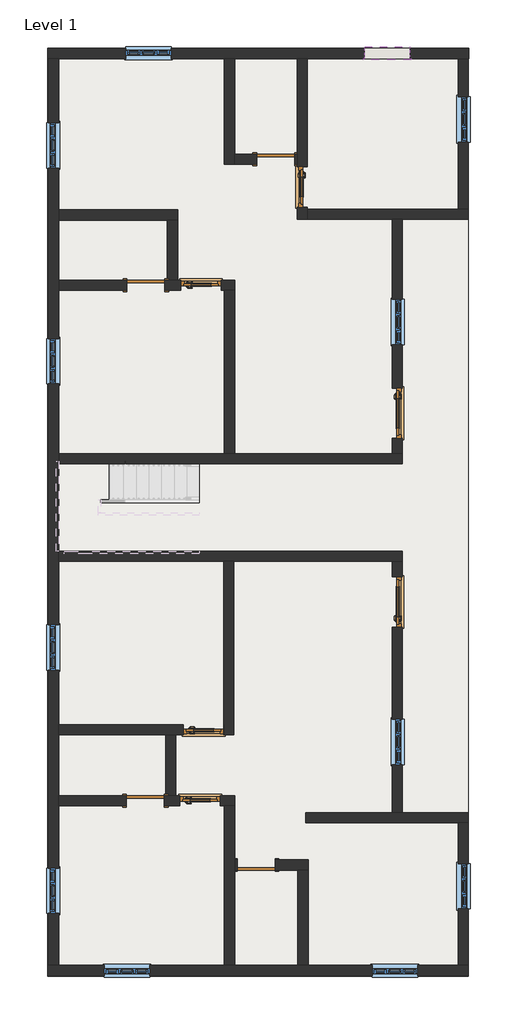
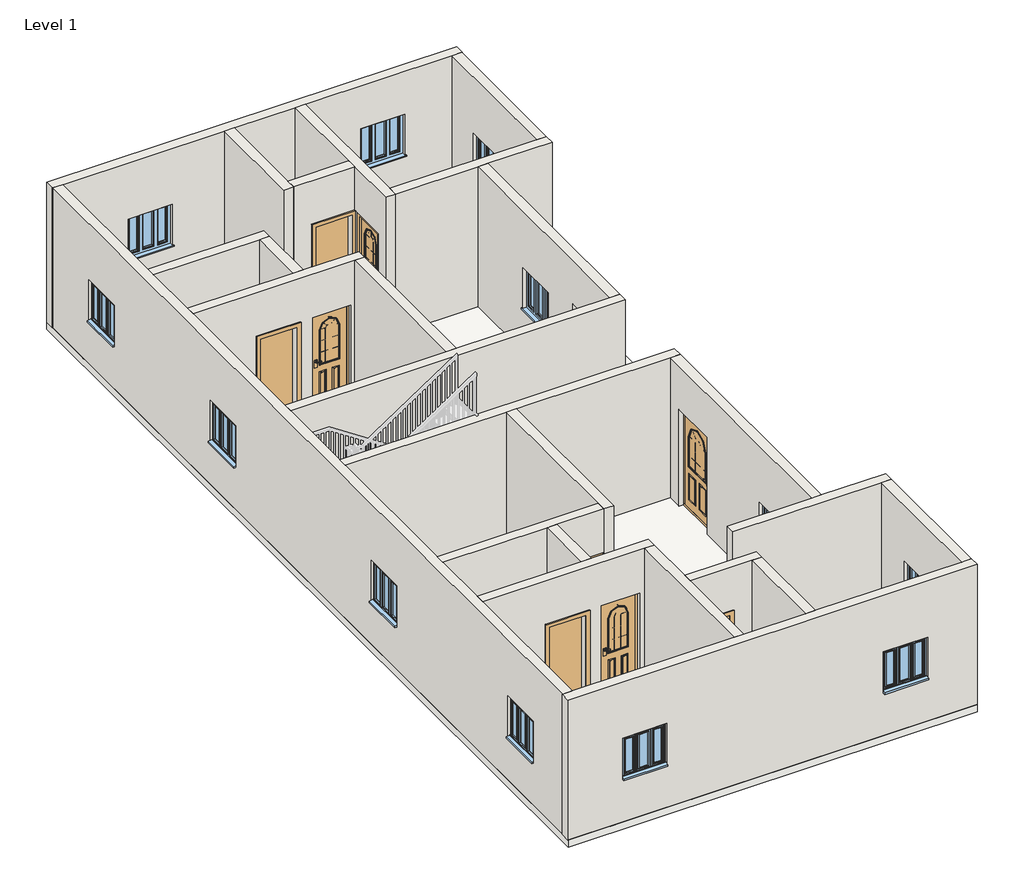
# One storey, part 1 of 2: 25 walls, 12 windows, 10 doors, 1 slab.
"""IFC4 building model written with IfcOpenShell, lengths in millimetres."""

from ifc_helpers import new_model, si_unit, frame, origin, origin_with_axes, place, context, project, spatial, polyline, outline, extrude, faceted_brep, transform, mapped, element, save
from components import doors_extsgl_w_glazing_bars_arched_1010x2110mm_bccdb1b2, doors_extsgl_w_glazing_bars_arched_1010x2110mm_5c897e1f, doors_extsgl_w_glazing_bars_arched_810x2110mm_57ea6d9e, doors_extsgl_w_glazing_bars_arched_810x2110mm_84a0a083, door_fadea3f2, windows_tpl_w_glazing_bars_910x910mm_9d987a72

model = new_model("IFC4")

# Units and contexts
model_context = context("Model", 3, world=origin())
ifc_project = project(units=[si_unit("LENGTHUNIT", "METRE", prefix="MILLI")], contexts=[model_context])

# Site, building, storey
site = spatial("IfcSite", under=ifc_project)
building = spatial("IfcBuilding", under=site)
storey = spatial("IfcBuildingStorey", under=building, Name="Level 1", Elevation=0.0)

# Doors
placement = place(None, origin())
doors_extsgl_w_glazing_bars_arched_1010x2110mm_shape = doors_extsgl_w_glazing_bars_arched_1010x2110mm_bccdb1b2(model_context)
element("IfcDoor", 1, ObjectType="Doors_ExtSgl_w-Glazing_Bars_Arched : 1010x2110mm", at=placement, inside=storey, context=model_context, shape_type="MappedRepresentation", body=[
    mapped(doors_extsgl_w_glazing_bars_arched_1010x2110mm_shape, transform((1850.5605895, 2208.5797121, 0.0), x_axis=(0.0, -1.0, 0.0), y_axis=(1.0, 0.0, 0.0), z_axis=(0.0, 0.0, 1.0))),
])
doors_extsgl_w_glazing_bars_arched_1010x2110mm_2_shape = doors_extsgl_w_glazing_bars_arched_1010x2110mm_5c897e1f(model_context)
element("IfcDoor", 2, ObjectType="Doors_ExtSgl_w-Glazing_Bars_Arched : 1010x2110mm", at=placement, inside=storey, context=model_context, shape_type="MappedRepresentation", body=[
    mapped(doors_extsgl_w_glazing_bars_arched_1010x2110mm_2_shape, transform((1850.5605895, -1576.0202879, 0.0), x_axis=(0.0, 1.0, 0.0), y_axis=(-1.0, 0.0, 0.0), z_axis=(0.0, 0.0, 1.0))),
])
doors_extsgl_w_glazing_bars_arched_810x2110mm_shape = doors_extsgl_w_glazing_bars_arched_810x2110mm_57ea6d9e(model_context)
element("IfcDoor", 3, ObjectType="Doors_ExtSgl_w-Glazing_Bars_Arched : 810x2110mm", at=placement, inside=storey, context=model_context, shape_type="MappedRepresentation", body=[
    mapped(doors_extsgl_w_glazing_bars_arched_810x2110mm_shape, transform((-2086.4394105, 4773.9797121, 0.0), x_axis=(1.0, 0.0, 0.0), y_axis=(0.0, 1.0, 0.0), z_axis=(0.0, 0.0, 1.0))),
])
element("IfcDoor", 4, ObjectType="Doors_ExtSgl_w-Glazing_Bars_Arched : 810x2110mm", at=placement, inside=storey, context=model_context, shape_type="MappedRepresentation", body=[
    mapped(doors_extsgl_w_glazing_bars_arched_810x2110mm_shape, transform((-2105.4894105, -5563.8202879, 0.0), x_axis=(1.0, 0.0, 0.0), y_axis=(0.0, 1.0, 0.0), z_axis=(0.0, 0.0, 1.0))),
])
doors_extsgl_w_glazing_bars_arched_810x2110mm_2_shape = doors_extsgl_w_glazing_bars_arched_810x2110mm_84a0a083(model_context)
element("IfcDoor", 5, ObjectType="Doors_ExtSgl_w-Glazing_Bars_Arched : 810x2110mm", at=placement, inside=storey, context=model_context, shape_type="MappedRepresentation", body=[
    mapped(doors_extsgl_w_glazing_bars_arched_810x2110mm_2_shape, transform((-2035.6394105, -4141.4202879, 0.0), x_axis=(1.0, 0.0, 0.0), y_axis=(0.0, 1.0, 0.0), z_axis=(0.0, 0.0, 1.0))),
])
element("IfcDoor", 6, ObjectType="Doors_ExtSgl_w-Glazing_Bars_Arched : 810x2110mm", at=placement, inside=storey, context=model_context, shape_type="MappedRepresentation", body=[
    mapped(doors_extsgl_w_glazing_bars_arched_810x2110mm_2_shape, transform((-54.4394105, 6748.5640518, 0.0), x_axis=(0.0, -1.0, 0.0), y_axis=(1.0, 0.0, 0.0), z_axis=(0.0, 0.0, 1.0))),
])
door_shape = door_fadea3f2(model_context)
element("IfcDoor", 7, ObjectType="Single-Flush : 30\" x 80\"", at=placement, inside=storey, context=model_context, shape_type="MappedRepresentation", body=[
    mapped(door_shape, transform((-3204.0394105, -5563.8202879, 0.0), x_axis=(1.0, 0.0, 0.0), y_axis=(0.0, 1.0, 0.0), z_axis=(0.0, 0.0, 1.0))),
])
element("IfcDoor", 8, ObjectType="Single-Flush : 30\" x 80\"", at=placement, inside=storey, context=model_context, shape_type="MappedRepresentation", body=[
    mapped(door_shape, transform((-981.5394105, -6850.9128362, 0.0), x_axis=(-1.0, 0.0, 0.0), y_axis=(0.0, -1.0, 0.0), z_axis=(0.0, 0.0, 1.0))),
])
element("IfcDoor", 9, ObjectType="Single-Flush : 30\" x 80\"", at=placement, inside=storey, context=model_context, shape_type="MappedRepresentation", body=[
    mapped(door_shape, transform((-3191.3394105, 4773.9797121, 0.0), x_axis=(1.0, 0.0, 0.0), y_axis=(0.0, 1.0, 0.0), z_axis=(0.0, 0.0, 1.0))),
])
element("IfcDoor", 10, ObjectType="Single-Flush : 30\" x 80\"", at=placement, inside=storey, context=model_context, shape_type="MappedRepresentation", body=[
    mapped(door_shape, transform((-587.8394105, 7301.2797121, 0.0), x_axis=(1.0, 0.0, 0.0), y_axis=(0.0, 1.0, 0.0), z_axis=(0.0, 0.0, 1.0))),
])

# Slab
element("IfcSlab", 11, ObjectType="Generic - 12\"", at=placement, inside=storey, context=model_context, shape_type="SweptSolid", body=[
    extrude(outline(polyline([(3272.9605895, 9523.7797121), (3272.9605895, -9081.7202879), (-5159.8394105, -9081.7202879), (-5159.8394105, 9523.7797121), (3272.9605895, 9523.7797121)])), frame((0.0, 0.0, -152.4), z_axis=(0.0, 0.0, 1.0), x_axis=(1.0, 0.0, 0.0)), (0.0, 0.0, 1.0), 152.4),
])

# Walls
element("IfcWall", 12, ObjectType="Generic - 4.5\" p", at=placement, inside=storey, context=model_context, shape_type="Brep", body=[
    faceted_brep([(-2810.3394105, 4672.3797121, 2032.0), (-2810.3394105, 4672.3797121, 0.0), (-2491.4394105, 4672.3797121, 0.0), (-2491.4394105, 4672.3797121, 2110.0), (-1681.4394105, 4672.3797121, 2110.0), (-1681.4394105, 4672.3797121, 0.0), (-1616.5394105, 4672.3797121, 0.0), (-1413.3394105, 4672.3797121, 0.0), (-1413.3394105, 4672.3797121, 3048.0), (-1616.5394105, 4672.3797121, 3048.0), (-4943.9394105, 4672.3797121, 3048.0), (-4943.9394105, 4672.3797121, 0.0), (-3572.3394105, 4672.3797121, 0.0), (-3572.3394105, 4672.3797121, 2032.0), (-2491.4394105, 4875.5797121, 0.0), (-2556.3394105, 4875.5797121, 0.0), (-2759.5394105, 4875.5797121, 0.0), (-2810.3394105, 4875.5797121, 0.0), (-2810.3394105, 4875.5797121, 2032.0), (-3572.3394105, 4875.5797121, 2032.0), (-3572.3394105, 4875.5797121, 0.0), (-4943.9394105, 4875.5797121, 0.0), (-4943.9394105, 4875.5797121, 3048.0), (-2759.5394105, 4875.5797121, 3048.0), (-2556.3394105, 4875.5797121, 3048.0), (-1413.3394105, 4875.5797121, 3048.0), (-1413.3394105, 4875.5797121, 0.0), (-1681.4394105, 4875.5797121, 0.0), (-1681.4394105, 4875.5797121, 2110.0), (-2491.4394105, 4875.5797121, 2110.0)], [[[0, 1, 2, 3, 4, 5, 6, 7, 8, 9, 10, 11, 12, 13]], [[14, 15, 16, 17, 18, 19, 20, 21, 22, 23, 24, 25, 26, 27, 28, 29]], [[7, 6, 5, 27, 26]], [[12, 11, 21, 20]], [[2, 1, 17, 16, 15, 14]], [[10, 9, 8, 25, 24, 23, 22]], [[11, 10, 22, 21]], [[8, 7, 26, 25]], [[14, 29, 3, 2]], [[28, 27, 5, 4]], [[29, 28, 4, 3]], [[18, 17, 1, 0]], [[19, 18, 0, 13]], [[20, 19, 13, 12]]]),
])
element("IfcWall", 13, ObjectType="Generic - 4.5\" p", at=placement, inside=storey, context=model_context, shape_type="SweptSolid", body=[
    extrude(outline(polyline([(-1616.5394105, 1395.7797121), (-1616.5394105, 4672.3797121), (-1413.3394105, 4672.3797121), (-1413.3394105, 1395.7797121), (-1616.5394105, 1395.7797121)])), origin_with_axes(), (0.0, 0.0, 1.0), 3048.0),
])
element("IfcWall", 14, ObjectType="Generic - 4.5\" p", at=placement, inside=storey, context=model_context, shape_type="Brep", body=[
    faceted_brep([(-4943.9394105, 6082.1542467, 0.0), (-2759.5394105, 6082.1542467, 0.0), (-2556.3394105, 6082.1542467, 0.0), (-2556.3394105, 6082.1542467, 3048.0), (-2759.5394105, 6082.1542467, 3048.0), (-4943.9394105, 6082.1542467, 3048.0), (-4943.9394105, 6285.3542467, 0.0), (-4943.9394105, 6285.3542467, 3048.0), (-2556.3394105, 6285.3542467, 3048.0), (-2556.3394105, 6285.3542467, 0.0)], [[[0, 1, 2, 3, 4, 5]], [[6, 7, 8, 9]], [[2, 1, 0, 6, 9]], [[5, 4, 3, 8, 7]], [[0, 5, 7, 6]], [[3, 2, 9, 8]]]),
])
element("IfcWall", 15, ObjectType="Generic - 4.5\" p", at=placement, inside=storey, context=model_context, shape_type="SweptSolid", body=[
    extrude(outline(polyline([(-2759.5394105, 4875.5797121), (-2759.5394105, 6082.1542467), (-2556.3394105, 6082.1542467), (-2556.3394105, 4875.5797121), (-2759.5394105, 4875.5797121)])), origin_with_axes(), (0.0, 0.0, 1.0), 3048.0),
])
element("IfcWall", 16, ObjectType="Generic - 4.5\" p", at=placement, inside=storey, context=model_context, shape_type="Brep", body=[
    faceted_brep([(-1616.5394105, 9320.5797121, 0.0), (-1616.5394105, 7199.6797121, 0.0), (-1616.5394105, 7199.6797121, 3048.0), (-1616.5394105, 9320.5797121, 3048.0), (-1413.3394105, 9320.5797121, 0.0), (-1413.3394105, 9320.5797121, 3048.0), (-1413.3394105, 7402.8797121, 3048.0), (-1413.3394105, 7199.6797121, 3048.0), (-1413.3394105, 7199.6797121, 0.0), (-1413.3394105, 7402.8797121, 0.0)], [[[0, 1, 2, 3]], [[4, 5, 6, 7, 8, 9]], [[1, 0, 4, 9, 8]], [[3, 2, 7, 6, 5]], [[0, 3, 5, 4]], [[2, 1, 8, 7]]]),
])
element("IfcWall", 17, ObjectType="Generic - 4.5\" p", at=placement, inside=storey, context=model_context, shape_type="SweptSolid", body=[
    extrude(outline(polyline([(2032.0, -206.8394105), (0.0, -206.8394105), (0.0, -156.0394105), (3048.0, -156.0394105), (3048.0, -1413.3394105), (0.0, -1413.3394105), (0.0, -968.8394105), (2032.0, -968.8394105), (2032.0, -206.8394105)])), frame((0.0, 7199.6797121, 0.0), z_axis=(0.0, 1.0, 0.0), x_axis=(0.0, 0.0, 1.0)), (0.0, 0.0, 1.0), 203.2),
])
element("IfcWall", 18, ObjectType="Generic - 4.5\" p", at=placement, inside=storey, context=model_context, shape_type="Brep", body=[
    faceted_brep([(-156.0394105, 6343.5640518, 2110.0), (-156.0394105, 6343.5640518, 0.0), (-156.0394105, 6094.2483916, 0.0), (-156.0394105, 6094.2483916, 3048.0), (-156.0394105, 7199.6797121, 3048.0), (-156.0394105, 7402.8797121, 3048.0), (-156.0394105, 9320.5797121, 3048.0), (-156.0394105, 9320.5797121, 0.0), (-156.0394105, 7402.8797121, 0.0), (-156.0394105, 7199.6797121, 0.0), (-156.0394105, 7153.5640518, 0.0), (-156.0394105, 7153.5640518, 2110.0), (47.1605895, 6094.2483916, 0.0), (47.1605895, 6297.4483916, 0.0), (47.1605895, 6343.5640518, 0.0), (47.1605895, 6343.5640518, 2110.0), (47.1605895, 7153.5640518, 2110.0), (47.1605895, 7153.5640518, 0.0), (47.1605895, 9320.5797121, 0.0), (47.1605895, 9320.5797121, 3048.0), (47.1605895, 6297.4483916, 3048.0), (47.1605895, 6094.2483916, 3048.0)], [[[0, 1, 2, 3, 4, 5, 6, 7, 8, 9, 10, 11]], [[12, 13, 14, 15, 16, 17, 18, 19, 20, 21]], [[2, 1, 14, 13, 12]], [[10, 9, 8, 7, 18, 17]], [[6, 5, 4, 3, 21, 20, 19]], [[7, 6, 19, 18]], [[3, 2, 12, 21]], [[17, 16, 11, 10]], [[15, 14, 1, 0]], [[16, 15, 0, 11]]]),
])
element("IfcWall", 19, ObjectType="Generic - 4.5\" p", at=placement, inside=storey, context=model_context, shape_type="Brep", body=[
    faceted_brep([(47.1605895, 6094.2483916, 0.0), (1748.9605895, 6094.2483916, 0.0), (1952.1605895, 6094.2483916, 0.0), (3272.9605895, 6094.2483916, 0.0), (3272.9605895, 6094.2483916, 3048.0), (1952.1605895, 6094.2483916, 3048.0), (1748.9605895, 6094.2483916, 3048.0), (47.1605895, 6094.2483916, 3048.0), (47.1605895, 6297.4483916, 0.0), (47.1605895, 6297.4483916, 3048.0), (3069.7605895, 6297.4483916, 3048.0), (3272.9605895, 6297.4483916, 3048.0), (3272.9605895, 6297.4483916, 0.0), (3069.7605895, 6297.4483916, 0.0)], [[[0, 1, 2, 3, 4, 5, 6, 7]], [[8, 9, 10, 11, 12, 13]], [[3, 2, 1, 0, 8, 13, 12]], [[7, 6, 5, 4, 11, 10, 9]], [[0, 7, 9, 8]], [[4, 3, 12, 11]]]),
])
element("IfcWall", 20, ObjectType="Generic - 4.5\" p", at=placement, inside=storey, context=model_context, shape_type="Brep", body=[
    faceted_brep([(-4943.9394105, 1192.5797121, 0.0), (1952.1605895, 1192.5797121, 0.0), (1952.1605895, 1192.5797121, 3048.0), (-4943.9394105, 1192.5797121, 3048.0), (-4943.9394105, 1395.7797121, 0.0), (-4943.9394105, 1395.7797121, 3048.0), (-1616.5394105, 1395.7797121, 3048.0), (-1413.3394105, 1395.7797121, 3048.0), (1748.9605895, 1395.7797121, 3048.0), (1952.1605895, 1395.7797121, 3048.0), (1952.1605895, 1395.7797121, 0.0), (1748.9605895, 1395.7797121, 0.0), (-1413.3394105, 1395.7797121, 0.0), (-1616.5394105, 1395.7797121, 0.0)], [[[0, 1, 2, 3]], [[4, 5, 6, 7, 8, 9, 10, 11, 12, 13]], [[1, 0, 4, 13, 12, 11, 10]], [[3, 2, 9, 8, 7, 6, 5]], [[0, 3, 5, 4]], [[2, 1, 10, 9]]]),
])
element("IfcWall", 21, ObjectType="Generic - 4.5\" p", at=placement, inside=storey, context=model_context, shape_type="Brep", body=[
    faceted_brep([(-4943.9394105, -763.2202879, 0.0), (-1629.2394105, -763.2202879, 0.0), (-1426.0394105, -763.2202879, 0.0), (1748.9605895, -763.2202879, 0.0), (1952.1605895, -763.2202879, 0.0), (1952.1605895, -763.2202879, 3048.0), (1748.9605895, -763.2202879, 3048.0), (-1426.0394105, -763.2202879, 3048.0), (-1629.2394105, -763.2202879, 3048.0), (-4943.9394105, -763.2202879, 3048.0), (-4943.9394105, -560.0202879, 0.0), (-4943.9394105, -560.0202879, 3048.0), (1952.1605895, -560.0202879, 3048.0), (1952.1605895, -560.0202879, 0.0)], [[[0, 1, 2, 3, 4, 5, 6, 7, 8, 9]], [[10, 11, 12, 13]], [[4, 3, 2, 1, 0, 10, 13]], [[9, 8, 7, 6, 5, 12, 11]], [[0, 9, 11, 10]], [[5, 4, 13, 12]]]),
])
element("IfcWall", 22, ObjectType="Generic - 4.5\" p", at=placement, inside=storey, context=model_context, shape_type="Brep", body=[
    faceted_brep([(-1629.2394105, -763.2202879, 0.0), (-1629.2394105, -4039.8202879, 0.0), (-1629.2394105, -4243.0202879, 0.0), (-1629.2394105, -4243.0202879, 3048.0), (-1629.2394105, -4039.8202879, 3048.0), (-1629.2394105, -763.2202879, 3048.0), (-1426.0394105, -763.2202879, 0.0), (-1426.0394105, -763.2202879, 3048.0), (-1426.0394105, -4243.0202879, 3048.0), (-1426.0394105, -4243.0202879, 0.0)], [[[0, 1, 2, 3, 4, 5]], [[6, 7, 8, 9]], [[2, 1, 0, 6, 9]], [[5, 4, 3, 8, 7]], [[0, 5, 7, 6]], [[3, 2, 9, 8]]]),
])
element("IfcWall", 23, ObjectType="Generic - 4.5\" p", at=placement, inside=storey, context=model_context, shape_type="Brep", body=[
    faceted_brep([(-1630.6394105, -4243.0202879, 2110.0), (-1630.6394105, -4243.0202879, 0.0), (-1629.2394105, -4243.0202879, 0.0), (-1629.2394105, -4243.0202879, 3048.0), (-2594.4394105, -4243.0202879, 3048.0), (-2797.6394105, -4243.0202879, 3048.0), (-4943.9394105, -4243.0202879, 3048.0), (-4943.9394105, -4243.0202879, 0.0), (-2797.6394105, -4243.0202879, 0.0), (-2594.4394105, -4243.0202879, 0.0), (-2440.6394105, -4243.0202879, 0.0), (-2440.6394105, -4243.0202879, 2110.0), (-1629.2394105, -4039.8202879, 0.0), (-1630.6394105, -4039.8202879, 0.0), (-1630.6394105, -4039.8202879, 2110.0), (-2440.6394105, -4039.8202879, 2110.0), (-2440.6394105, -4039.8202879, 0.0), (-4943.9394105, -4039.8202879, 0.0), (-4943.9394105, -4039.8202879, 3048.0), (-1629.2394105, -4039.8202879, 3048.0)], [[[0, 1, 2, 3, 4, 5, 6, 7, 8, 9, 10, 11]], [[12, 13, 14, 15, 16, 17, 18, 19]], [[2, 1, 13, 12]], [[10, 9, 8, 7, 17, 16]], [[6, 5, 4, 3, 19, 18]], [[3, 2, 12, 19]], [[7, 6, 18, 17]], [[16, 15, 11, 10]], [[14, 13, 1, 0]], [[15, 14, 0, 11]]]),
])
element("IfcWall", 24, ObjectType="Generic - 4.5\" p", at=placement, inside=storey, context=model_context, shape_type="Brep", body=[
    faceted_brep([(-2823.0394105, -5665.4202879, 2032.0), (-2823.0394105, -5665.4202879, 0.0), (-2510.4894105, -5665.4202879, 0.0), (-2510.4894105, -5665.4202879, 2110.0), (-1700.4894105, -5665.4202879, 2110.0), (-1700.4894105, -5665.4202879, 0.0), (-1616.5394105, -5665.4202879, 0.0), (-1413.3394105, -5665.4202879, 0.0), (-1413.3394105, -5665.4202879, 3048.0), (-1616.5394105, -5665.4202879, 3048.0), (-4943.9394105, -5665.4202879, 3048.0), (-4943.9394105, -5665.4202879, 0.0), (-3585.0394105, -5665.4202879, 0.0), (-3585.0394105, -5665.4202879, 2032.0), (-2510.4894105, -5462.2202879, 0.0), (-2594.4394105, -5462.2202879, 0.0), (-2797.6394105, -5462.2202879, 0.0), (-2823.0394105, -5462.2202879, 0.0), (-2823.0394105, -5462.2202879, 2032.0), (-3585.0394105, -5462.2202879, 2032.0), (-3585.0394105, -5462.2202879, 0.0), (-4943.9394105, -5462.2202879, 0.0), (-4943.9394105, -5462.2202879, 3048.0), (-2797.6394105, -5462.2202879, 3048.0), (-2594.4394105, -5462.2202879, 3048.0), (-1413.3394105, -5462.2202879, 3048.0), (-1413.3394105, -5462.2202879, 0.0), (-1700.4894105, -5462.2202879, 0.0), (-1700.4894105, -5462.2202879, 2110.0), (-2510.4894105, -5462.2202879, 2110.0)], [[[0, 1, 2, 3, 4, 5, 6, 7, 8, 9, 10, 11, 12, 13]], [[14, 15, 16, 17, 18, 19, 20, 21, 22, 23, 24, 25, 26, 27, 28, 29]], [[7, 6, 5, 27, 26]], [[12, 11, 21, 20]], [[2, 1, 17, 16, 15, 14]], [[10, 9, 8, 25, 24, 23, 22]], [[11, 10, 22, 21]], [[8, 7, 26, 25]], [[14, 29, 3, 2]], [[28, 27, 5, 4]], [[29, 28, 4, 3]], [[18, 17, 1, 0]], [[19, 18, 0, 13]], [[20, 19, 13, 12]]]),
])
element("IfcWall", 25, ObjectType="Generic - 4.5\" p", at=placement, inside=storey, context=model_context, shape_type="SweptSolid", body=[
    extrude(outline(polyline([(-2797.6394105, -5462.2202879), (-2797.6394105, -4243.0202879), (-2594.4394105, -4243.0202879), (-2594.4394105, -5462.2202879), (-2797.6394105, -5462.2202879)])), origin_with_axes(), (0.0, 0.0, 1.0), 3048.0),
])
element("IfcWall", 26, ObjectType="Generic - 4.5\" p", at=placement, inside=storey, context=model_context, shape_type="Brep", body=[
    faceted_brep([(-1616.5394105, -5665.4202879, 0.0), (-1616.5394105, -8865.8202879, 0.0), (-1616.5394105, -8865.8202879, 3048.0), (-1616.5394105, -5665.4202879, 3048.0), (-1413.3394105, -5665.4202879, 0.0), (-1413.3394105, -5665.4202879, 3048.0), (-1413.3394105, -6749.3128362, 3048.0), (-1413.3394105, -6952.5128362, 3048.0), (-1413.3394105, -8865.8202879, 3048.0), (-1413.3394105, -8865.8202879, 0.0), (-1413.3394105, -6952.5128362, 0.0), (-1413.3394105, -6749.3128362, 0.0)], [[[0, 1, 2, 3]], [[4, 5, 6, 7, 8, 9, 10, 11]], [[1, 0, 4, 11, 10, 9]], [[3, 2, 8, 7, 6, 5]], [[0, 3, 5, 4]], [[2, 1, 9, 8]]]),
])
element("IfcWall", 27, ObjectType="Generic - 4.5\" p", at=placement, inside=storey, context=model_context, shape_type="Brep", body=[
    faceted_brep([(-1413.3394105, -6952.5128362, 0.0), (-1362.5394105, -6952.5128362, 0.0), (-1362.5394105, -6952.5128362, 2032.0), (-600.5394105, -6952.5128362, 2032.0), (-600.5394105, -6952.5128362, 0.0), (-143.3394105, -6952.5128362, 0.0), (59.8605895, -6952.5128362, 0.0), (59.8605895, -6952.5128362, 3048.0), (-143.3394105, -6952.5128362, 3048.0), (-1413.3394105, -6952.5128362, 3048.0), (-1362.5394105, -6749.3128362, 2032.0), (-1362.5394105, -6749.3128362, 0.0), (-1413.3394105, -6749.3128362, 0.0), (-1413.3394105, -6749.3128362, 3048.0), (59.8605895, -6749.3128362, 3048.0), (59.8605895, -6749.3128362, 0.0), (-600.5394105, -6749.3128362, 0.0), (-600.5394105, -6749.3128362, 2032.0)], [[[0, 1, 2, 3, 4, 5, 6, 7, 8, 9]], [[10, 11, 12, 13, 14, 15, 16, 17]], [[16, 15, 6, 5, 4]], [[12, 11, 1, 0]], [[9, 8, 7, 14, 13]], [[0, 9, 13, 12]], [[7, 6, 15, 14]], [[2, 1, 11, 10]], [[3, 2, 10, 17]], [[4, 3, 17, 16]]]),
])
element("IfcWall", 28, ObjectType="Generic - 4.5\" p", at=placement, inside=storey, context=model_context, shape_type="SweptSolid", body=[
    extrude(outline(polyline([(-143.3394105, -8865.8202879), (-143.3394105, -6952.5128362), (59.8605895, -6952.5128362), (59.8605895, -8865.8202879), (-143.3394105, -8865.8202879)])), origin_with_axes(), (0.0, 0.0, 1.0), 3048.0),
])
element("IfcWall", 29, ObjectType="Generic - 4.5\" p", at=placement, inside=storey, context=model_context, shape_type="Brep", body=[
    faceted_brep([(3272.9605895, -5805.1202879, 0.0), (1952.1605895, -5805.1202879, 0.0), (1748.9605895, -5805.1202879, 0.0), (9.0605895, -5805.1202879, 0.0), (9.0605895, -5805.1202879, 3048.0), (1748.9605895, -5805.1202879, 3048.0), (1952.1605895, -5805.1202879, 3048.0), (3272.9605895, -5805.1202879, 3048.0), (3272.9605895, -6008.3202879, 0.0), (3272.9605895, -6008.3202879, 3048.0), (3069.7605895, -6008.3202879, 3048.0), (9.0605895, -6008.3202879, 3048.0), (9.0605895, -6008.3202879, 0.0), (3069.7605895, -6008.3202879, 0.0)], [[[0, 1, 2, 3, 4, 5, 6, 7]], [[8, 9, 10, 11, 12, 13]], [[3, 2, 1, 0, 8, 13, 12]], [[4, 3, 12, 11]], [[7, 6, 5, 4, 11, 10, 9]], [[0, 7, 9, 8]]]),
])
element("IfcWall", 30, ObjectType="Generic - 9\" w", at=placement, inside=storey, context=model_context, shape_type="Brep", body=[
    faceted_brep([(-5159.8394105, 9320.5797121, 0.0), (-5147.1394105, 9320.5797121, 0.0), (-4943.9394105, 9320.5797121, 0.0), (-1616.5394105, 9320.5797121, 0.0), (-1413.3394105, 9320.5797121, 0.0), (-156.0394105, 9320.5797121, 0.0), (47.1605895, 9320.5797121, 0.0), (3069.7605895, 9320.5797121, 0.0), (3272.9605895, 9320.5797121, 0.0), (3285.6605895, 9320.5797121, 0.0), (3285.6605895, 9320.5797121, 3048.0), (3272.9605895, 9320.5797121, 3048.0), (3069.7605895, 9320.5797121, 3048.0), (47.1605895, 9320.5797121, 3048.0), (-156.0394105, 9320.5797121, 3048.0), (-1413.3394105, 9320.5797121, 3048.0), (-1616.5394105, 9320.5797121, 3048.0), (-4943.9394105, 9320.5797121, 3048.0), (-5147.1394105, 9320.5797121, 3048.0), (-5159.8394105, 9320.5797121, 3048.0), (1192.3605895, 9320.5797121, 2110.0), (2102.3605895, 9320.5797121, 2110.0), (2102.3605895, 9320.5797121, 1200.0), (1192.3605895, 9320.5797121, 1200.0), (-3595.5394105, 9320.5797121, 1824.4), (-2685.5394105, 9320.5797121, 1824.4), (-2685.5394105, 9320.5797121, 914.4), (-3595.5394105, 9320.5797121, 914.4), (-5159.8394105, 9523.7797121, 0.0), (-5159.8394105, 9523.7797121, 3048.0), (3285.6605895, 9523.7797121, 3048.0), (3285.6605895, 9523.7797121, 0.0), (1192.3605895, 9523.7797121, 2110.0), (1192.3605895, 9523.7797121, 1200.0), (2102.3605895, 9523.7797121, 1200.0), (2102.3605895, 9523.7797121, 2110.0), (-3595.5394105, 9523.7797121, 1824.4), (-3595.5394105, 9523.7797121, 914.4), (-2685.5394105, 9523.7797121, 914.4), (-2685.5394105, 9523.7797121, 1824.4)], [[[0, 1, 2, 3, 4, 5, 6, 7, 8, 9, 10, 11, 12, 13, 14, 15, 16, 17, 18, 19], [20, 21, 22, 23], [24, 25, 26, 27]], [[28, 29, 30, 31], [32, 33, 34, 35], [36, 37, 38, 39]], [[9, 8, 7, 6, 5, 4, 3, 2, 1, 0, 28, 31]], [[10, 9, 31, 30]], [[19, 18, 17, 16, 15, 14, 13, 12, 11, 10, 30, 29]], [[0, 19, 29, 28]], [[33, 32, 20, 23]], [[34, 33, 23, 22]], [[35, 34, 22, 21]], [[32, 35, 21, 20]], [[37, 36, 24, 27]], [[38, 37, 27, 26]], [[39, 38, 26, 25]], [[36, 39, 25, 24]]]),
])
element("IfcWall", 31, ObjectType="Generic - 9\" w", at=placement, inside=storey, context=model_context, shape_type="Brep", body=[
    faceted_brep([(3272.9605895, -8865.8202879, 0.0), (3069.7605895, -8865.8202879, 0.0), (59.8605895, -8865.8202879, 0.0), (-143.3394105, -8865.8202879, 0.0), (-1413.3394105, -8865.8202879, 0.0), (-1616.5394105, -8865.8202879, 0.0), (-4943.9394105, -8865.8202879, 0.0), (-5147.1394105, -8865.8202879, 0.0), (-5159.8394105, -8865.8202879, 0.0), (-5159.8394105, -8865.8202879, 3048.0), (-5147.1394105, -8865.8202879, 3048.0), (-4943.9394105, -8865.8202879, 3048.0), (-1616.5394105, -8865.8202879, 3048.0), (-1413.3394105, -8865.8202879, 3048.0), (-143.3394105, -8865.8202879, 3048.0), (59.8605895, -8865.8202879, 3048.0), (3069.7605895, -8865.8202879, 3048.0), (3272.9605895, -8865.8202879, 3048.0), (-3117.3394105, -8865.8202879, 1824.4), (-4027.3394105, -8865.8202879, 1824.4), (-4027.3394105, -8865.8202879, 914.4), (-3117.3394105, -8865.8202879, 914.4), (2254.7605895, -8865.8202879, 1824.4), (1344.7605895, -8865.8202879, 1824.4), (1344.7605895, -8865.8202879, 914.4), (2254.7605895, -8865.8202879, 914.4), (3272.9605895, -9069.0202879, 0.0), (3272.9605895, -9069.0202879, 3048.0), (-5159.8394105, -9069.0202879, 3048.0), (-5159.8394105, -9069.0202879, 0.0), (-3117.3394105, -9069.0202879, 1824.4), (-3117.3394105, -9069.0202879, 914.4), (-4027.3394105, -9069.0202879, 914.4), (-4027.3394105, -9069.0202879, 1824.4), (2254.7605895, -9069.0202879, 1824.4), (2254.7605895, -9069.0202879, 914.4), (1344.7605895, -9069.0202879, 914.4), (1344.7605895, -9069.0202879, 1824.4)], [[[0, 1, 2, 3, 4, 5, 6, 7, 8, 9, 10, 11, 12, 13, 14, 15, 16, 17], [18, 19, 20, 21], [22, 23, 24, 25]], [[26, 27, 28, 29], [30, 31, 32, 33], [34, 35, 36, 37]], [[8, 7, 6, 5, 4, 3, 2, 1, 0, 26, 29]], [[9, 8, 29, 28]], [[17, 16, 15, 14, 13, 12, 11, 10, 9, 28, 27]], [[0, 17, 27, 26]], [[31, 30, 18, 21]], [[32, 31, 21, 20]], [[33, 32, 20, 19]], [[30, 33, 19, 18]], [[35, 34, 22, 25]], [[36, 35, 25, 24]], [[37, 36, 24, 23]], [[34, 37, 23, 22]]]),
])
element("IfcWall", 32, ObjectType="Generic - 9\" w", at=placement, inside=storey, context=model_context, shape_type="Brep", body=[
    faceted_brep([(-4943.9394105, -8865.8202879, 0.0), (-4943.9394105, -5665.4202879, 0.0), (-4943.9394105, -5462.2202879, 0.0), (-4943.9394105, -4243.0202879, 0.0), (-4943.9394105, -4039.8202879, 0.0), (-4943.9394105, -763.2202879, 0.0), (-4943.9394105, -560.0202879, 0.0), (-4943.9394105, 1192.5797121, 0.0), (-4943.9394105, 1395.7797121, 0.0), (-4943.9394105, 4672.3797121, 0.0), (-4943.9394105, 4875.5797121, 0.0), (-4943.9394105, 6082.1542467, 0.0), (-4943.9394105, 6285.3542467, 0.0), (-4943.9394105, 9320.5797121, 0.0), (-4943.9394105, 9320.5797121, 3048.0), (-4943.9394105, 6285.3542467, 3048.0), (-4943.9394105, 6082.1542467, 3048.0), (-4943.9394105, 4875.5797121, 3048.0), (-4943.9394105, 4672.3797121, 3048.0), (-4943.9394105, 1395.7797121, 3048.0), (-4943.9394105, 1192.5797121, 3048.0), (-4943.9394105, -560.0202879, 3048.0), (-4943.9394105, -763.2202879, 3048.0), (-4943.9394105, -4039.8202879, 3048.0), (-4943.9394105, -4243.0202879, 3048.0), (-4943.9394105, -5462.2202879, 3048.0), (-4943.9394105, -5665.4202879, 3048.0), (-4943.9394105, -8865.8202879, 3048.0), (-4943.9394105, -7822.2202879, 1824.4), (-4943.9394105, -6912.2202879, 1824.4), (-4943.9394105, -6912.2202879, 914.4), (-4943.9394105, -7822.2202879, 914.4), (-4943.9394105, -2945.4202879, 1824.4), (-4943.9394105, -2035.4202879, 1824.4), (-4943.9394105, -2035.4202879, 914.4), (-4943.9394105, -2945.4202879, 914.4), (-4943.9394105, 2794.9797121, 1824.4), (-4943.9394105, 3704.9797121, 1824.4), (-4943.9394105, 3704.9797121, 914.4), (-4943.9394105, 2794.9797121, 914.4), (-4943.9394105, 7125.7542467, 1824.4), (-4943.9394105, 8035.7542467, 1824.4), (-4943.9394105, 8035.7542467, 914.4), (-4943.9394105, 7125.7542467, 914.4), (-5147.1394105, -8865.8202879, 0.0), (-5147.1394105, -8865.8202879, 3048.0), (-5147.1394105, 9320.5797121, 3048.0), (-5147.1394105, 9320.5797121, 0.0), (-5147.1394105, -7822.2202879, 1824.4), (-5147.1394105, -7822.2202879, 914.4), (-5147.1394105, -6912.2202879, 914.4), (-5147.1394105, -6912.2202879, 1824.4), (-5147.1394105, -2945.4202879, 1824.4), (-5147.1394105, -2945.4202879, 914.4), (-5147.1394105, -2035.4202879, 914.4), (-5147.1394105, -2035.4202879, 1824.4), (-5147.1394105, 2794.9797121, 1824.4), (-5147.1394105, 2794.9797121, 914.4), (-5147.1394105, 3704.9797121, 914.4), (-5147.1394105, 3704.9797121, 1824.4), (-5147.1394105, 7125.7542467, 1824.4), (-5147.1394105, 7125.7542467, 914.4), (-5147.1394105, 8035.7542467, 914.4), (-5147.1394105, 8035.7542467, 1824.4)], [[[0, 1, 2, 3, 4, 5, 6, 7, 8, 9, 10, 11, 12, 13, 14, 15, 16, 17, 18, 19, 20, 21, 22, 23, 24, 25, 26, 27], [28, 29, 30, 31], [32, 33, 34, 35], [36, 37, 38, 39], [40, 41, 42, 43]], [[44, 45, 46, 47], [48, 49, 50, 51], [52, 53, 54, 55], [56, 57, 58, 59], [60, 61, 62, 63]], [[13, 12, 11, 10, 9, 8, 7, 6, 5, 4, 3, 2, 1, 0, 44, 47]], [[27, 26, 25, 24, 23, 22, 21, 20, 19, 18, 17, 16, 15, 14, 46, 45]], [[14, 13, 47, 46]], [[0, 27, 45, 44]], [[49, 48, 28, 31]], [[50, 49, 31, 30]], [[51, 50, 30, 29]], [[48, 51, 29, 28]], [[53, 52, 32, 35]], [[54, 53, 35, 34]], [[55, 54, 34, 33]], [[52, 55, 33, 32]], [[57, 56, 36, 39]], [[58, 57, 39, 38]], [[59, 58, 38, 37]], [[56, 59, 37, 36]], [[61, 60, 40, 43]], [[62, 61, 43, 42]], [[63, 62, 42, 41]], [[60, 63, 41, 40]]]),
])
element("IfcWall", 33, ObjectType="Generic - 9\" w", at=placement, inside=storey, context=model_context, shape_type="SweptSolid", body=[
    extrude(outline(polyline([(-8865.8202879, 0.0), (-8865.8202879, 3048.0), (-6008.3202879, 3048.0), (-6008.3202879, 0.0), (-8865.8202879, 0.0)]), holes=[polyline([(-6823.3202879, 1824.4), (-7733.3202879, 1824.4), (-7733.3202879, 914.4), (-6823.3202879, 914.4), (-6823.3202879, 1824.4)])]), frame((3069.7605895, 0.0, 0.0), z_axis=(1.0, 0.0, 0.0), x_axis=(0.0, 1.0, 0.0)), (0.0, 0.0, 1.0), 203.2),
])
element("IfcWall", 34, ObjectType="Generic - 9\" w", at=placement, inside=storey, context=model_context, shape_type="SweptSolid", body=[
    extrude(outline(polyline([(9320.5797121, 0.0), (6297.4483916, 0.0), (6297.4483916, 3048.0), (9320.5797121, 3048.0), (9320.5797121, 0.0)]), holes=[polyline([(8556.3797121, 1824.4), (7646.3797121, 1824.4), (7646.3797121, 914.4), (8556.3797121, 914.4), (8556.3797121, 1824.4)])]), frame((3069.7605895, 0.0, 0.0), z_axis=(1.0, 0.0, 0.0), x_axis=(0.0, 1.0, 0.0)), (0.0, 0.0, 1.0), 203.2),
])
element("IfcWall", 35, ObjectType="Generic - 9\" w", at=placement, inside=storey, context=model_context, shape_type="SweptSolid", body=[
    extrude(outline(polyline([(-763.2202879, 0.0), (-1071.0202879, 0.0), (-1071.0202879, 2110.0), (-2081.0202879, 2110.0), (-2081.0202879, 0.0), (-5805.1202879, 0.0), (-5805.1202879, 3048.0), (-763.2202879, 3048.0), (-763.2202879, 0.0)]), holes=[polyline([(-3927.7202879, 1824.4), (-4837.7202879, 1824.4), (-4837.7202879, 914.4), (-3927.7202879, 914.4), (-3927.7202879, 1824.4)])]), frame((1748.9605895, 0.0, 0.0), z_axis=(1.0, 0.0, 0.0), x_axis=(0.0, 1.0, 0.0)), (0.0, 0.0, 1.0), 203.2),
])
element("IfcWall", 36, ObjectType="Generic - 9\" w", at=placement, inside=storey, context=model_context, shape_type="SweptSolid", body=[
    extrude(outline(polyline([(1703.5797121, 2110.0), (1703.5797121, 0.0), (1395.7797121, 0.0), (1395.7797121, 3048.0), (6094.2483916, 3048.0), (6094.2483916, 0.0), (2713.5797121, 0.0), (2713.5797121, 2110.0), (1703.5797121, 2110.0)]), holes=[polyline([(4492.3797121, 1824.4), (3582.3797121, 1824.4), (3582.3797121, 914.4), (4492.3797121, 914.4), (4492.3797121, 1824.4)])]), frame((1748.9605895, 0.0, 0.0), z_axis=(1.0, 0.0, 0.0), x_axis=(0.0, 1.0, 0.0)), (0.0, 0.0, 1.0), 203.2),
])

# Windows
windows_tpl_w_glazing_bars_910x910mm_shape = windows_tpl_w_glazing_bars_910x910mm_9d987a72(model_context)
element("IfcWindow", 37, ObjectType="Windows_Tpl_w-Glazing_Bars : 910x910mm", at=placement, inside=storey, context=model_context, shape_type="MappedRepresentation", body=[
    mapped(windows_tpl_w_glazing_bars_910x910mm_shape, transform((-3809.0060772, -8958.9637201, -285.6), x_axis=(-1.0, 0.0, 0.0), y_axis=(0.0, -1.0, 0.0), z_axis=(0.0, 0.0, 1.0))),
])
element("IfcWindow", 38, ObjectType="Windows_Tpl_w-Glazing_Bars : 910x910mm", at=placement, inside=storey, context=model_context, shape_type="MappedRepresentation", body=[
    mapped(windows_tpl_w_glazing_bars_910x910mm_shape, transform((-5037.0828427, -7130.5536213, -285.6), x_axis=(0.0, 1.0, 0.0), y_axis=(-1.0, 0.0, 0.0), z_axis=(0.0, 0.0, 1.0))),
])
element("IfcWindow", 39, ObjectType="Windows_Tpl_w-Glazing_Bars : 910x910mm", at=placement, inside=storey, context=model_context, shape_type="MappedRepresentation", body=[
    mapped(windows_tpl_w_glazing_bars_910x910mm_shape, transform((-5037.0828427, -2253.7536213, -285.6), x_axis=(0.0, 1.0, 0.0), y_axis=(-1.0, 0.0, 0.0), z_axis=(0.0, 0.0, 1.0))),
])
element("IfcWindow", 40, ObjectType="Windows_Tpl_w-Glazing_Bars : 910x910mm", at=placement, inside=storey, context=model_context, shape_type="MappedRepresentation", body=[
    mapped(windows_tpl_w_glazing_bars_910x910mm_shape, transform((-5037.0828427, 3486.6463787, -285.6), x_axis=(0.0, 1.0, 0.0), y_axis=(-1.0, 0.0, 0.0), z_axis=(0.0, 0.0, 1.0))),
])
element("IfcWindow", 41, ObjectType="Windows_Tpl_w-Glazing_Bars : 910x910mm", at=placement, inside=storey, context=model_context, shape_type="MappedRepresentation", body=[
    mapped(windows_tpl_w_glazing_bars_910x910mm_shape, transform((3162.9040216, 7864.7130454, -285.6), x_axis=(0.0, -1.0, 0.0), y_axis=(1.0, 0.0, 0.0), z_axis=(0.0, 0.0, 1.0))),
])
element("IfcWindow", 42, ObjectType="Windows_Tpl_w-Glazing_Bars : 910x910mm", at=placement, inside=storey, context=model_context, shape_type="MappedRepresentation", body=[
    mapped(windows_tpl_w_glazing_bars_910x910mm_shape, transform((1884.0272561, 9413.7231443, 0.0), x_axis=(1.0, 0.0, 0.0), y_axis=(0.0, 1.0, 0.0), z_axis=(0.0, 0.0, 1.0))),
])
element("IfcWindow", 43, ObjectType="Windows_Tpl_w-Glazing_Bars : 910x910mm", at=placement, inside=storey, context=model_context, shape_type="MappedRepresentation", body=[
    mapped(windows_tpl_w_glazing_bars_910x910mm_shape, transform((1563.0939228, -8958.9637201, -285.6), x_axis=(-1.0, 0.0, 0.0), y_axis=(0.0, -1.0, 0.0), z_axis=(0.0, 0.0, 1.0))),
])
element("IfcWindow", 44, ObjectType="Windows_Tpl_w-Glazing_Bars : 910x910mm", at=placement, inside=storey, context=model_context, shape_type="MappedRepresentation", body=[
    mapped(windows_tpl_w_glazing_bars_910x910mm_shape, transform((3162.9040216, -7514.9869546, -285.6), x_axis=(0.0, -1.0, 0.0), y_axis=(1.0, 0.0, 0.0), z_axis=(0.0, 0.0, 1.0))),
])
element("IfcWindow", 45, ObjectType="Windows_Tpl_w-Glazing_Bars : 910x910mm", at=placement, inside=storey, context=model_context, shape_type="MappedRepresentation", body=[
    mapped(windows_tpl_w_glazing_bars_910x910mm_shape, transform((-5037.0828427, 7817.4209133, -285.6), x_axis=(0.0, 1.0, 0.0), y_axis=(-1.0, 0.0, 0.0), z_axis=(0.0, 0.0, 1.0))),
])
element("IfcWindow", 46, ObjectType="Windows_Tpl_w-Glazing_Bars : 910x910mm", at=placement, inside=storey, context=model_context, shape_type="MappedRepresentation", body=[
    mapped(windows_tpl_w_glazing_bars_910x910mm_shape, transform((-2903.8727439, 9413.7231443, -285.6), x_axis=(1.0, 0.0, 0.0), y_axis=(0.0, 1.0, 0.0), z_axis=(0.0, 0.0, 1.0))),
])
element("IfcWindow", 47, ObjectType="Windows_Tpl_w-Glazing_Bars : 910x910mm", at=placement, inside=storey, context=model_context, shape_type="MappedRepresentation", body=[
    mapped(windows_tpl_w_glazing_bars_910x910mm_shape, transform((1842.1040216, -4619.3869546, -285.6), x_axis=(0.0, -1.0, 0.0), y_axis=(1.0, 0.0, 0.0), z_axis=(0.0, 0.0, 1.0))),
])
element("IfcWindow", 48, ObjectType="Windows_Tpl_w-Glazing_Bars : 910x910mm", at=placement, inside=storey, context=model_context, shape_type="MappedRepresentation", body=[
    mapped(windows_tpl_w_glazing_bars_910x910mm_shape, transform((1842.1040216, 3800.7130454, -285.6), x_axis=(0.0, -1.0, 0.0), y_axis=(1.0, 0.0, 0.0), z_axis=(0.0, 0.0, 1.0))),
])

save(model, "model.ifc")

# Revit data of these elements
# Type "Doors_ExtSgl_w-Glazing_Bars_Arched : 1010x2110mm"
#   Type Mark = "10"
#   Type Comments = "External Single"
#   Operation = "SingleSwingRight"
#   Construction Type Id = "SGL"
#   Keynote = "L20"
#   Analytic Construction = "Large single-glazed windows"
#   Wrap Layers (Int) from Ext = 177.5 mm
#   Wrap Layers (Ext) from Ext = 102.5 mm
#   Visual Light Transmittance = 0.9
#   Thickness = 44 mm
#   Solar Heat Gain Coefficient = 0.86
#   Rough Width = 1010 mm
#   Rough Height = 2110 mm
#   O/A Frame Width = 64 mm
#   Heat Transfer Coefficient (U) = 0.979472 BTU/(h·ft²·°F)
#   Handle Z Distance = 1050 mm
#   Glazing Thickness = 24 mm
#   FrameWidth = 42 mm
#   FrameOffset - External = 25 mm
#   FrameDepth = 89 mm
#   Door Panel Width = 907 mm
#   Door Panel Thickness = 44 mm
#   Door Panel Height = 2000 mm
#   DONT CHANGE - Half Glazed Width = 303.5 mm
#   DONT CHANGE - Glazed Width = 607 mm
#   Cill Thickness = 54.5 mm
#   Cill Projection = 30 mm
#   Handle X Distance = 75 mm
#   Height = 2110 mm
#   Structural Tolerance = 6.5 mm
#   Tolerance = 3 mm
#   Undercut = 4 mm
#   Width = 1010 mm
#   Cill Extension = 25 mm
#   Cavity Closer Width = 50 mm
#   Cavity Closer Offset from Ext = 102.5 mm
#   Cavity Closer Depth = 85 mm
#   Vis - Ironmongery = yes
#   Vis - Glazing Bars = yes
#   Vis - Cavity Closers = yes
#   Define Thermal Properties by = 1
#   Function = 1
#   Material Glass = Door - Glazing
#   Material Glazing Bar = Door - Panel
#   Material Door = Door - Panel
#   Material Frame = Door - Frame/Mullion
#   Material Ironmongery = Door - Handle
#   Wall Closure = (empty or 0)
# Type "Doors_ExtSgl_w-Glazing_Bars_Arched : 810x2110mm"
#   Type Mark = "9"
#   Type Comments = "External Single"
#   Operation = "SingleSwingRight"
#   Construction Type Id = "SGL"
#   Keynote = "L20"
#   Analytic Construction = "Large single-glazed windows"
#   Wrap Layers (Int) from Ext = 177.5 mm
#   Wrap Layers (Ext) from Ext = 102.5 mm
#   Visual Light Transmittance = 0.9
#   Thickness = 44 mm
#   Solar Heat Gain Coefficient = 0.86
#   Rough Width = 810 mm
#   Rough Height = 2110 mm
#   O/A Frame Width = 64 mm
#   Heat Transfer Coefficient (U) = 0.979472 BTU/(h·ft²·°F)
#   Handle Z Distance = 1050 mm
#   Glazing Thickness = 24 mm
#   FrameWidth = 42 mm
#   FrameOffset - External = 25 mm
#   FrameDepth = 89 mm
#   Door Panel Width = 707 mm
#   Door Panel Thickness = 44 mm
#   Door Panel Height = 2000 mm
#   DONT CHANGE - Half Glazed Width = 203.5 mm
#   DONT CHANGE - Glazed Width = 407 mm
#   Cill Thickness = 54.5 mm
#   Cill Projection = 30 mm
#   Handle X Distance = 75 mm
#   Height = 2110 mm
#   Structural Tolerance = 6.5 mm
#   Tolerance = 3 mm
#   Undercut = 4 mm
#   Width = 810 mm
#   Cill Extension = 25 mm
#   Cavity Closer Width = 50 mm
#   Cavity Closer Offset from Ext = 102.5 mm
#   Cavity Closer Depth = 85 mm
#   Vis - Ironmongery = yes
#   Vis - Glazing Bars = yes
#   Vis - Cavity Closers = yes
#   Define Thermal Properties by = 1
#   Function = 1
#   Material Glass = Door - Glazing
#   Material Glazing Bar = Door - Panel
#   Material Door = Door - Panel
#   Material Frame = Door - Frame/Mullion
#   Material Ironmongery = Door - Handle
#   Wall Closure = (empty or 0)
# Type "Single-Flush : 30\" x 80\""
#   Type Mark = "5"
#   Construction Type Id = "MDOOR"
#   Assembly Code = "C1020"
#   Analytic Construction = "Metal"
#   Thickness = 50.8 mm
#   Heat Transfer Coefficient (U) = 0.651978 BTU/(h·ft²·°F)
#   Height = 2032 mm
#   Trim Projection Ext = 25.4 mm
#   Trim Projection Int = 25.4 mm
#   Trim Width = 76.2 mm
#   Width = 762 mm
#   Define Thermal Properties by = 1
#   Define Thermal Properties by = 1
#   Door Material = Door - Panel
#   Frame Material = Door - Frame
#   Visual Light Transmittance = 0
#   Solar Heat Gain Coefficient = 0
#   Function = (empty or 0)
#   Wall Closure = (empty or 0)
# Type "Generic - 12\""
#   Assembly Code = "B1010"
#   Function = 0
#   Layers, outside or top first: 152.4 mm no material (function 1)
# Type "Generic - 4.5\" p"
#   Assembly Code = "B2010"
#   Layers, outside or top first: 203.2 mm no material (function 1)
# Type "Generic - 9\" w"
#   Assembly Code = "B2010"
#   Layers, outside or top first: 203.2 mm no material (function 1)
# Type "Windows_Tpl_w-Glazing_Bars : 910x910mm"
#   Type Mark = "18"
#   Operation = "TriplePanelVertical"
#   Construction Type Id = "GSP4R"
#   Manufacturer = "Revit"
#   Keynote = "L10"
#   Analytic Construction = "1/8 in Pilkington single glazing"
#   Length 1 = 24 mm
#   Wrap Layers (Ext) from Ext = 102.5 mm
#   Wrap Layers (Int) from Ext = 177.5 mm
#   Window Board Projection = 25 mm
#   Window Board Extension = 25 mm
#   Visual Light Transmittance = 0.9
#   Solar Heat Gain Coefficient = 0.78
#   Rough Width = 910 mm
#   Rough Height = 910 mm
#   Height = 910 mm
#   Width = 910 mm
#   Heat Transfer Coefficient (U) = 0.6496 BTU/(h·ft²·°F)
#   Glazing Thickness = 24 mm
#   Glazing Bar Thickness = 20 mm
#   FrameOffset - External = 50 mm
#   Frame Depth = 65 mm
#   Default Head Height = 2110 mm
#   Cill Depth = 87.5 mm
#   Cavity Closer Width = 50 mm
#   Cavity Closer Offset from Ext = 102.5 mm
#   Cavity Closer Depth = 85 mm
#   Vis - Glazing Bars = yes
#   Vis - Cavity Closers = yes
#   Define Thermal Properties by = 1
#   Material Trim = Window Frame
#   Material Glazing Bars = Window Frame
#   Material Glass = Glass
#   Material Frame = Window Frame
#   Wall Closure = (empty or 0)
# Elements 1, 2 (IfcDoor, "Doors_ExtSgl_w-Glazing_Bars_Arched : 1010x2110mm")
#   Phase Created = New Construction
#   Materials on its faces: "Door - Panel", "Door - Handle", "Door - Frame/Mullion", "Door - Glazing"
# Elements 3, 4, 5, 6 (IfcDoor, "Doors_ExtSgl_w-Glazing_Bars_Arched : 810x2110mm")
#   Phase Created = New Construction
#   Materials on its faces: "Door - Panel", "Door - Handle", "Door - Frame/Mullion", "Door - Glazing"
# Elements 7, 8, 9, 10 (IfcDoor, "Single-Flush : 30\" x 80\"")
#   Phase Created = New Construction
#   Materials on its faces: "Door - Frame", "Door - Panel"
# Element 11 (IfcSlab, "Generic - 12\"")
#   Height Offset From Level = 0 mm
#   Phase Created = New Construction
#   Materials on its faces: "Default Floor", "Wood Planks", "Door - Frame", "Default Mass Interior Wall"
# Elements 12, 13, 14, 15, 16, 17, 18, 22, 23, 24, 25, 26, 27, 28 (IfcWall, "Generic - 4.5\" p")
#   Top Offset = 0 mm
#   Base Offset = 0 mm
#   wall height = 3048 mm
#   Phase Created = New Construction
#   Base Constraint = Level 1
#   Top Constraint = Level 2
#   Materials on its faces: "Default Wall"
# Elements 19, 29 (IfcWall, "Generic - 4.5\" p")
#   Top Offset = 0 mm
#   Base Offset = 0 mm
#   wall height = 3048 mm
#   Phase Created = New Construction
#   Base Constraint = Level 1
#   Top Constraint = Level 2
#   Materials on its faces: "Default Wall", "Default Mass Interior Wall"
# Elements 20, 21 (IfcWall, "Generic - 4.5\" p")
#   Top Offset = 0 mm
#   Base Offset = 0 mm
#   wall height = 3048 mm
#   Phase Created = New Construction
#   Base Constraint = Level 1
#   Top Constraint = Level 2
#   Materials on its faces: "Default Wall", "Window Frame", "Wood Planks"
# Elements 30, 31 (IfcWall, "Generic - 9\" w")
#   Top Offset = 0 mm
#   Base Offset = 0 mm
#   wall height = 3048 mm
#   Phase Created = New Construction
#   Base Constraint = Level 1
#   Top Constraint = Level 2
#   Materials on its faces: "Default Wall", "Wood Planks", "Default Mass Interior Wall"
# Elements 32, 35, 36 (IfcWall, "Generic - 9\" w")
#   Top Offset = 0 mm
#   Base Offset = 0 mm
#   wall height = 3048 mm
#   Phase Created = New Construction
#   Base Constraint = Level 1
#   Top Constraint = Level 2
#   Materials on its faces: "Default Wall", "Wood Planks"
# Elements 33, 34 (IfcWall, "Generic - 9\" w")
#   Top Offset = 0 mm
#   Base Offset = 0 mm
#   wall height = 3048 mm
#   Phase Created = New Construction
#   Base Constraint = Level 1
#   Top Constraint = Level 2
#   Materials on its faces: "Default Wall", "Default Mass Interior Wall"
# Element 37 (IfcWindow, "Windows_Tpl_w-Glazing_Bars : 910x910mm")
#   Mark = "1"
#   Phase Created = New Construction
#   Materials on its faces: "Window Frame", "Glass"
# Element 38 (IfcWindow, "Windows_Tpl_w-Glazing_Bars : 910x910mm")
#   Mark = "2"
#   Phase Created = New Construction
#   Materials on its faces: "Window Frame", "Glass"
# Element 39 (IfcWindow, "Windows_Tpl_w-Glazing_Bars : 910x910mm")
#   Mark = "3"
#   Phase Created = New Construction
#   Materials on its faces: "Window Frame", "Glass"
# Element 40 (IfcWindow, "Windows_Tpl_w-Glazing_Bars : 910x910mm")
#   Mark = "4"
#   Phase Created = New Construction
#   Materials on its faces: "Window Frame", "Glass"
# Element 41 (IfcWindow, "Windows_Tpl_w-Glazing_Bars : 910x910mm")
#   Mark = "5"
#   Phase Created = New Construction
#   Materials on its faces: "Window Frame", "Glass"
# Element 42 (IfcWindow, "Windows_Tpl_w-Glazing_Bars : 910x910mm")
#   Mark = "6"
#   Phase Created = New Construction
#   Materials on its faces: "Window Frame", "Glass"
# Element 43 (IfcWindow, "Windows_Tpl_w-Glazing_Bars : 910x910mm")
#   Mark = "9"
#   Phase Created = New Construction
#   Materials on its faces: "Window Frame", "Glass"
# Element 44 (IfcWindow, "Windows_Tpl_w-Glazing_Bars : 910x910mm")
#   Mark = "10"
#   Phase Created = New Construction
#   Materials on its faces: "Window Frame", "Glass"
# Element 45 (IfcWindow, "Windows_Tpl_w-Glazing_Bars : 910x910mm")
#   Mark = "12"
#   Phase Created = New Construction
#   Materials on its faces: "Window Frame", "Glass"
# Element 46 (IfcWindow, "Windows_Tpl_w-Glazing_Bars : 910x910mm")
#   Mark = "13"
#   Phase Created = New Construction
#   Materials on its faces: "Window Frame", "Glass"
# Element 47 (IfcWindow, "Windows_Tpl_w-Glazing_Bars : 910x910mm")
#   Mark = "14"
#   Phase Created = New Construction
#   Materials on its faces: "Window Frame", "Glass"
# Element 48 (IfcWindow, "Windows_Tpl_w-Glazing_Bars : 910x910mm")
#   Mark = "15"
#   Phase Created = New Construction
#   Materials on its faces: "Window Frame", "Glass"
# Materials
#   "Door - Glazing": colour RGB 0 0 255, transparency 0.75
#   "Door - Panel": class "Wood", colour RGB 210 159 95, transparency 0, Cost = 0
#   "Door - Frame/Mullion": class "Wood", colour RGB 212 179 113, transparency 0
#   "Door - Handle": colour RGB 246 240 166, transparency 0
#   "Door - Frame": colour RGB 118 70 51, transparency 0, Cost = 0
#   "Window Frame": colour RGB 249 249 249, transparency 0
#   "Glass": class "Glass", colour RGB 0 128 192, transparency 0.75, Description = "Soda Lime Glass", Cost = 0
#   "Default Floor": colour RGB 128 128 128, transparency 0, Cost = 0
#   "Wood Planks": class "Wood", colour RGB 193 160 115, transparency 0, Description = "Physical material.", Cost = 0
#   "Default Mass Interior Wall": class "Generic", colour RGB 195 229 126, transparency 0, Cost = 0
#   "Default Wall": colour RGB 128 128 128, transparency 0, Cost = 0
